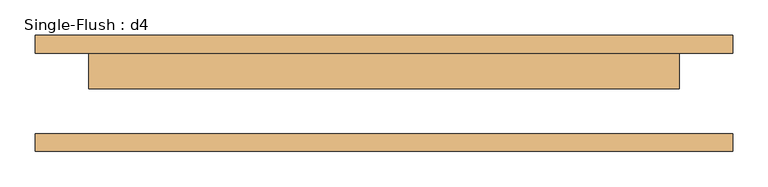
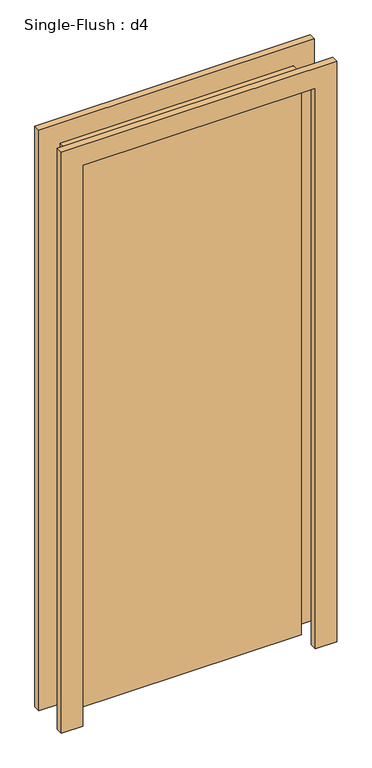
"""IFC4 building model written with IfcOpenShell, lengths in millimetres: door geometry, Single-Flush : d4."""

from ifc_helpers import new_model, si_unit, frame, origin, origin_with_axes, place, context, project, spatial, polyline, outline, extrude, source, transform, mapped, element, save


def single_flush_d4_f1814d11(model_context):
    return source(origin(), model_context, "Body", "SweptSolid", [
        extrude(outline(polyline([(2209.8, -495.3), (0.0, -495.3), (0.0, -419.1), (2133.6, -419.1), (2133.6, 419.1), (0.0, 419.1), (0.0, 495.3), (2209.8, 495.3), (2209.8, -495.3)])), frame((0.0, 57.15, 0.0), z_axis=(0.0, 1.0, 0.0), x_axis=(0.0, 0.0, 1.0)), (0.0, 0.0, 1.0), 25.4),
        extrude(outline(polyline([(2209.8, 495.3), (2209.8, -495.3), (0.0, -495.3), (0.0, -419.1), (2133.6, -419.1), (2133.6, 419.1), (0.0, 419.1), (0.0, 495.3), (2209.8, 495.3)])), frame((0.0, -82.55, 0.0), z_axis=(0.0, 1.0, 0.0), x_axis=(0.0, 0.0, 1.0)), (0.0, 0.0, 1.0), 25.4),
        extrude(outline(polyline([(419.1, 6.35), (-419.1, 6.35), (-419.1, 57.15), (419.1, 57.15), (419.1, 6.35)])), origin_with_axes(), (0.0, 0.0, 1.0), 2133.6),
    ])


if __name__ == "__main__":
    model = new_model("IFC4")
    model_context = context("Model", 3, world=origin())
    ifc_project = project(units=[si_unit("LENGTHUNIT", "METRE", prefix="MILLI")], contexts=[model_context])
    site = spatial("IfcSite", under=ifc_project)
    building = spatial("IfcBuilding", under=site)
    placement = place(None, origin())
    single_flush_d4_shape = single_flush_d4_f1814d11(model_context)
    element("IfcDoor", 1, ObjectType="Single-Flush : d4", at=placement, inside=building, context=model_context, shape_type="MappedRepresentation", body=[
        mapped(single_flush_d4_shape, transform((0.0, 0.0, 0.0), x_axis=(1.0, 0.0, 0.0), y_axis=(0.0, 1.0, 0.0), z_axis=(0.0, 0.0, 1.0))),
    ])
    save(model, "model.ifc")

# Revit data of these elements
# Type "Single-Flush : d4"
#   Type Mark = "11"
#   Construction Type Id = "MDOOR"
#   Assembly Code = "C1020"
#   Analytic Construction = "Metal"
#   Thickness = 0' - 2"
#   Heat Transfer Coefficient (U) = 0.651978 BTU/(h·ft²·°F)
#   Height = 7' - 0"
#   Trim Projection Ext = 0' - 1"
#   Trim Projection Int = 0' - 1"
#   Trim Width = 0' - 3"
#   Width = 2' - 9"
#   Define Thermal Properties by = 1
#   Door Material = Door - Panel
#   Frame Material = Door - Frame
#   Visual Light Transmittance = 0
#   Solar Heat Gain Coefficient = 0
#   Function = (empty or 0)
#   Wall Closure = (empty or 0)
# Element 1 (IfcDoor, "Single-Flush : d4")
#   Materials on its faces: "Door - Frame", "Door - Panel"
# Materials
#   "Door - Panel": class "Wood", colour RGB 210 159 95, transparency 0, Cost = 0
#   "Door - Frame": colour RGB 118 70 51, transparency 0, Cost = 0
